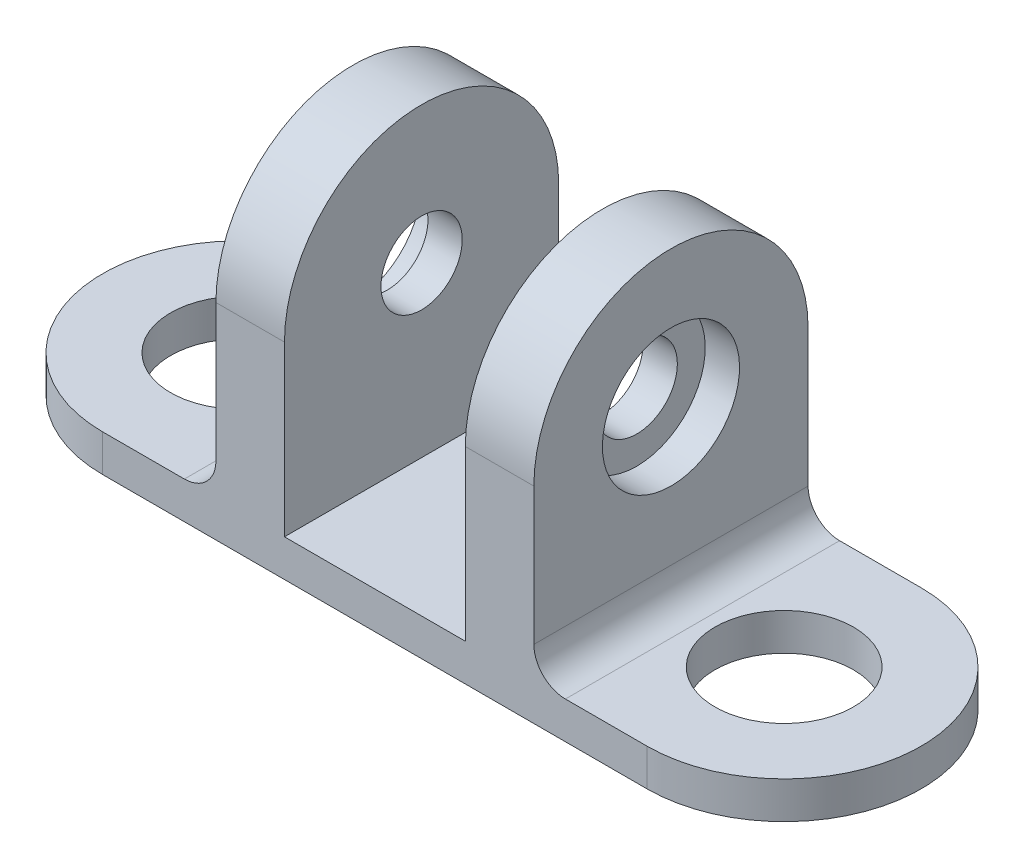
ISO-10303-21;
HEADER;
FILE_DESCRIPTION(('STEP AP214'),'2;1');
FILE_NAME('part.step','',(''),(''),'','','');
FILE_SCHEMA(('AUTOMOTIVE_DESIGN { 1 0 10303 214 1 1 1 1 }'));
ENDSEC;
DATA;
#1=APPLICATION_CONTEXT('core data for automotive mechanical design processes');
#2=APPLICATION_PROTOCOL_DEFINITION('international standard','automotive_design',2000,#1);
#3=PRODUCT_CONTEXT('',#1,'mechanical');
#4=PRODUCT('Part','Part','',(#3));
#5=PRODUCT_RELATED_PRODUCT_CATEGORY('part','',(#4));
#6=PRODUCT_DEFINITION_FORMATION('','',#4);
#7=PRODUCT_DEFINITION_CONTEXT('part definition',#1,'design');
#8=PRODUCT_DEFINITION('design','',#6,#7);
#9=PRODUCT_DEFINITION_SHAPE('','',#8);
#10=(LENGTH_UNIT() NAMED_UNIT(*) SI_UNIT(.MILLI.,.METRE.));
#11=(NAMED_UNIT(*) PLANE_ANGLE_UNIT() SI_UNIT($,.RADIAN.));
#12=(NAMED_UNIT(*) SI_UNIT($,.STERADIAN.) SOLID_ANGLE_UNIT());
#13=UNCERTAINTY_MEASURE_WITH_UNIT(LENGTH_MEASURE(1.E-05),#10,'distance_accuracy_value','');
#14=(GEOMETRIC_REPRESENTATION_CONTEXT(3) GLOBAL_UNCERTAINTY_ASSIGNED_CONTEXT((#13)) GLOBAL_UNIT_ASSIGNED_CONTEXT((#10,
#11,#12)) REPRESENTATION_CONTEXT('',''));
#15=CARTESIAN_POINT('',(0.,0.,0.));
#16=DIRECTION('',(0.,0.,1.));
#17=DIRECTION('',(1.,0.,0.));
#18=AXIS2_PLACEMENT_3D('',#15,#16,#17);
#19=CARTESIAN_POINT('',(-14.9812864248725,15.,0.));
#20=DIRECTION('',(1.,0.,0.));
#21=DIRECTION('',(0.,1.,0.));
#22=AXIS2_PLACEMENT_3D('',#19,#20,#21);
#23=CYLINDRICAL_SURFACE('',#22,2.965);
#24=CARTESIAN_POINT('',(6.595,15.,0.));
#25=DIRECTION('',(-1.,0.,0.));
#26=DIRECTION('',(0.,0.,1.));
#27=AXIS2_PLACEMENT_3D('',#24,#25,#26);
#28=CIRCLE('',#27,2.965);
#29=CARTESIAN_POINT('',(6.595,15.,2.965));
#30=VERTEX_POINT('',#29);
#31=EDGE_CURVE('E267',#30,#30,#28,.T.);
#32=ORIENTED_EDGE('',*,*,#31,.T.);
#33=EDGE_LOOP('',(#32));
#34=FACE_BOUND('',#33,.T.);
#35=CARTESIAN_POINT('',(9.095,15.,0.));
#36=DIRECTION('',(1.,0.,0.));
#37=DIRECTION('',(0.,1.,0.));
#38=AXIS2_PLACEMENT_3D('',#35,#36,#37);
#39=CIRCLE('',#38,2.965);
#40=CARTESIAN_POINT('',(9.095,17.965,0.));
#41=VERTEX_POINT('',#40);
#42=EDGE_CURVE('E43',#41,#41,#39,.T.);
#43=ORIENTED_EDGE('',*,*,#42,.T.);
#44=EDGE_LOOP('',(#43));
#45=FACE_BOUND('',#44,.T.);
#46=ADVANCED_FACE('F39',(#34,#45),#23,.F.);
#47=CARTESIAN_POINT('',(1.79128642487246,15.,0.));
#48=DIRECTION('',(-1.,0.,0.));
#49=DIRECTION('',(0.,-1.,0.));
#50=AXIS2_PLACEMENT_3D('',#47,#48,#49);
#51=CYLINDRICAL_SURFACE('',#50,2.965);
#52=CARTESIAN_POINT('',(-6.595,15.,0.));
#53=DIRECTION('',(1.,0.,0.));
#54=DIRECTION('',(0.,0.,-1.));
#55=AXIS2_PLACEMENT_3D('',#52,#53,#54);
#56=CIRCLE('',#55,2.965);
#57=CARTESIAN_POINT('',(-6.595,15.,-2.965));
#58=VERTEX_POINT('',#57);
#59=EDGE_CURVE('E155',#58,#58,#56,.F.);
#60=ORIENTED_EDGE('',*,*,#59,.F.);
#61=EDGE_LOOP('',(#60));
#62=FACE_BOUND('',#61,.T.);
#63=CARTESIAN_POINT('',(-9.095,15.,0.));
#64=DIRECTION('',(-1.,0.,0.));
#65=DIRECTION('',(0.,-1.,0.));
#66=AXIS2_PLACEMENT_3D('',#63,#64,#65);
#67=CIRCLE('',#66,2.965);
#68=CARTESIAN_POINT('',(-9.095,12.035,0.));
#69=VERTEX_POINT('',#68);
#70=EDGE_CURVE('E258',#69,#69,#67,.F.);
#71=ORIENTED_EDGE('',*,*,#70,.F.);
#72=EDGE_LOOP('',(#71));
#73=FACE_BOUND('',#72,.T.);
#74=ADVANCED_FACE('F313',(#62,#73),#51,.F.);
#75=CARTESIAN_POINT('',(-19.85,2.7,0.));
#76=DIRECTION('',(0.,1.,0.));
#77=DIRECTION('',(0.,0.,1.));
#78=AXIS2_PLACEMENT_3D('',#75,#76,#77);
#79=PLANE('',#78);
#80=DIRECTION('',(-1.,0.,0.));
#81=VECTOR('',#80,1.);
#82=CARTESIAN_POINT('',(-19.85,2.7,-10.));
#83=LINE('',#82,#81);
#84=CARTESIAN_POINT('',(19.85,2.7,-10.));
#85=VERTEX_POINT('',#84);
#86=CARTESIAN_POINT('',(13.895,2.7,-10.));
#87=VERTEX_POINT('',#86);
#88=EDGE_CURVE('E222',#85,#87,#83,.T.);
#89=ORIENTED_EDGE('',*,*,#88,.T.);
#90=DIRECTION('',(0.,0.,1.));
#91=VECTOR('',#90,1.);
#92=CARTESIAN_POINT('',(13.895,2.7,10.));
#93=LINE('',#92,#91);
#94=CARTESIAN_POINT('',(13.895,2.7,10.));
#95=VERTEX_POINT('',#94);
#96=EDGE_CURVE('E243',#87,#95,#93,.T.);
#97=ORIENTED_EDGE('',*,*,#96,.T.);
#98=DIRECTION('',(1.,0.,0.));
#99=VECTOR('',#98,1.);
#100=CARTESIAN_POINT('',(-19.85,2.7,10.));
#101=LINE('',#100,#99);
#102=CARTESIAN_POINT('',(19.85,2.7,10.));
#103=VERTEX_POINT('',#102);
#104=EDGE_CURVE('E213',#95,#103,#101,.T.);
#105=ORIENTED_EDGE('',*,*,#104,.T.);
#106=CARTESIAN_POINT('',(19.85,2.7,0.));
#107=DIRECTION('',(0.,1.,0.));
#108=DIRECTION('',(0.,0.,1.));
#109=AXIS2_PLACEMENT_3D('',#106,#107,#108);
#110=CIRCLE('',#109,10.);
#111=EDGE_CURVE('E220',#103,#85,#110,.T.);
#112=ORIENTED_EDGE('',*,*,#111,.T.);
#113=EDGE_LOOP('',(#89,#97,#105,#112));
#114=FACE_BOUND('',#113,.T.);
#115=CARTESIAN_POINT('',(19.85,2.7,0.));
#116=DIRECTION('',(0.,1.,0.));
#117=DIRECTION('',(0.,0.,1.));
#118=AXIS2_PLACEMENT_3D('',#115,#116,#117);
#119=CIRCLE('',#118,5.05);
#120=CARTESIAN_POINT('',(19.85,2.7,-5.05));
#121=VERTEX_POINT('',#120);
#122=EDGE_CURVE('E196',#121,#121,#119,.T.);
#123=ORIENTED_EDGE('',*,*,#122,.F.);
#124=EDGE_LOOP('',(#123));
#125=FACE_BOUND('',#124,.T.);
#126=ADVANCED_FACE('F317',(#114,#125),#79,.T.);
#127=DIRECTION('',(0.,0.,1.));
#128=VECTOR('',#127,1.);
#129=CARTESIAN_POINT('',(6.595,2.7,-23.2774244490413));
#130=LINE('',#129,#128);
#131=CARTESIAN_POINT('',(6.595,2.7,-10.));
#132=VERTEX_POINT('',#131);
#133=CARTESIAN_POINT('',(6.595,2.7,10.));
#134=VERTEX_POINT('',#133);
#135=EDGE_CURVE('E163',#132,#134,#130,.T.);
#136=ORIENTED_EDGE('',*,*,#135,.F.);
#137=CARTESIAN_POINT('',(-6.595,2.7,-10.));
#138=VERTEX_POINT('',#137);
#139=EDGE_CURVE('E223',#132,#138,#83,.T.);
#140=ORIENTED_EDGE('',*,*,#139,.T.);
#141=DIRECTION('',(0.,0.,1.));
#142=VECTOR('',#141,1.);
#143=CARTESIAN_POINT('',(-6.595,2.7,-23.2774244490413));
#144=LINE('',#143,#142);
#145=CARTESIAN_POINT('',(-6.595,2.7,10.));
#146=VERTEX_POINT('',#145);
#147=EDGE_CURVE('E184',#138,#146,#144,.T.);
#148=ORIENTED_EDGE('',*,*,#147,.T.);
#149=EDGE_CURVE('E217',#146,#134,#101,.T.);
#150=ORIENTED_EDGE('',*,*,#149,.T.);
#151=EDGE_LOOP('',(#136,#140,#148,#150));
#152=FACE_BOUND('',#151,.T.);
#153=ADVANCED_FACE('F358',(#152),#79,.T.);
#154=CARTESIAN_POINT('',(-19.85,2.7,10.));
#155=VERTEX_POINT('',#154);
#156=CARTESIAN_POINT('',(-13.895,2.7,10.));
#157=VERTEX_POINT('',#156);
#158=EDGE_CURVE('E214',#155,#157,#101,.T.);
#159=ORIENTED_EDGE('',*,*,#158,.T.);
#160=DIRECTION('',(0.,0.,1.));
#161=VECTOR('',#160,1.);
#162=CARTESIAN_POINT('',(-13.895,2.7,-10.));
#163=LINE('',#162,#161);
#164=CARTESIAN_POINT('',(-13.895,2.7,-10.));
#165=VERTEX_POINT('',#164);
#166=EDGE_CURVE('E62',#157,#165,#163,.F.);
#167=ORIENTED_EDGE('',*,*,#166,.T.);
#168=CARTESIAN_POINT('',(-19.85,2.7,-10.));
#169=VERTEX_POINT('',#168);
#170=EDGE_CURVE('E219',#165,#169,#83,.T.);
#171=ORIENTED_EDGE('',*,*,#170,.T.);
#172=CARTESIAN_POINT('',(-19.85,2.7,0.));
#173=DIRECTION('',(0.,1.,0.));
#174=DIRECTION('',(0.,0.,1.));
#175=AXIS2_PLACEMENT_3D('',#172,#173,#174);
#176=CIRCLE('',#175,10.);
#177=EDGE_CURVE('E209',#169,#155,#176,.T.);
#178=ORIENTED_EDGE('',*,*,#177,.T.);
#179=EDGE_LOOP('',(#159,#167,#171,#178));
#180=FACE_BOUND('',#179,.T.);
#181=CARTESIAN_POINT('',(-19.85,2.7,0.));
#182=DIRECTION('',(0.,1.,0.));
#183=DIRECTION('',(0.,0.,1.));
#184=AXIS2_PLACEMENT_3D('',#181,#182,#183);
#185=CIRCLE('',#184,5.05);
#186=CARTESIAN_POINT('',(-19.85,2.7,-5.05));
#187=VERTEX_POINT('',#186);
#188=EDGE_CURVE('E204',#187,#187,#185,.T.);
#189=ORIENTED_EDGE('',*,*,#188,.F.);
#190=EDGE_LOOP('',(#189));
#191=FACE_BOUND('',#190,.T.);
#192=ADVANCED_FACE('F352',(#180,#191),#79,.T.);
#193=CARTESIAN_POINT('',(-19.85,0.,0.));
#194=DIRECTION('',(0.,1.,0.));
#195=DIRECTION('',(0.,0.,1.));
#196=AXIS2_PLACEMENT_3D('',#193,#194,#195);
#197=PLANE('',#196);
#198=CARTESIAN_POINT('',(-19.85,0.,0.));
#199=DIRECTION('',(0.,1.,0.));
#200=DIRECTION('',(0.,0.,1.));
#201=AXIS2_PLACEMENT_3D('',#198,#199,#200);
#202=CIRCLE('',#201,10.);
#203=CARTESIAN_POINT('',(-19.85,0.,-10.));
#204=VERTEX_POINT('',#203);
#205=CARTESIAN_POINT('',(-19.85,0.,10.));
#206=VERTEX_POINT('',#205);
#207=EDGE_CURVE('E210',#204,#206,#202,.T.);
#208=ORIENTED_EDGE('',*,*,#207,.F.);
#209=DIRECTION('',(-1.,0.,0.));
#210=VECTOR('',#209,1.);
#211=CARTESIAN_POINT('',(-19.85,0.,-10.));
#212=LINE('',#211,#210);
#213=CARTESIAN_POINT('',(19.85,0.,-10.));
#214=VERTEX_POINT('',#213);
#215=EDGE_CURVE('E212',#214,#204,#212,.T.);
#216=ORIENTED_EDGE('',*,*,#215,.F.);
#217=CARTESIAN_POINT('',(19.85,0.,0.));
#218=DIRECTION('',(0.,1.,0.));
#219=DIRECTION('',(0.,0.,1.));
#220=AXIS2_PLACEMENT_3D('',#217,#218,#219);
#221=CIRCLE('',#220,10.);
#222=CARTESIAN_POINT('',(19.85,0.,10.));
#223=VERTEX_POINT('',#222);
#224=EDGE_CURVE('E230',#223,#214,#221,.T.);
#225=ORIENTED_EDGE('',*,*,#224,.F.);
#226=DIRECTION('',(1.,0.,0.));
#227=VECTOR('',#226,1.);
#228=CARTESIAN_POINT('',(-19.85,0.,10.));
#229=LINE('',#228,#227);
#230=EDGE_CURVE('E229',#206,#223,#229,.T.);
#231=ORIENTED_EDGE('',*,*,#230,.F.);
#232=EDGE_LOOP('',(#208,#216,#225,#231));
#233=FACE_BOUND('',#232,.T.);
#234=CARTESIAN_POINT('',(-19.85,0.,0.));
#235=DIRECTION('',(0.,1.,0.));
#236=DIRECTION('',(0.,0.,1.));
#237=AXIS2_PLACEMENT_3D('',#234,#235,#236);
#238=CIRCLE('',#237,5.05);
#239=CARTESIAN_POINT('',(-19.85,0.,-5.05));
#240=VERTEX_POINT('',#239);
#241=EDGE_CURVE('E203',#240,#240,#238,.T.);
#242=ORIENTED_EDGE('',*,*,#241,.T.);
#243=EDGE_LOOP('',(#242));
#244=FACE_BOUND('',#243,.T.);
#245=CARTESIAN_POINT('',(19.85,0.,0.));
#246=DIRECTION('',(0.,1.,0.));
#247=DIRECTION('',(0.,0.,1.));
#248=AXIS2_PLACEMENT_3D('',#245,#246,#247);
#249=CIRCLE('',#248,5.05);
#250=CARTESIAN_POINT('',(19.85,0.,-5.05));
#251=VERTEX_POINT('',#250);
#252=EDGE_CURVE('E197',#251,#251,#249,.T.);
#253=ORIENTED_EDGE('',*,*,#252,.T.);
#254=EDGE_LOOP('',(#253));
#255=FACE_BOUND('',#254,.T.);
#256=ADVANCED_FACE('F355',(#233,#244,#255),#197,.F.);
#257=CARTESIAN_POINT('',(-19.85,2.7,0.));
#258=DIRECTION('',(0.,-1.,0.));
#259=DIRECTION('',(0.,0.,-1.));
#260=AXIS2_PLACEMENT_3D('',#257,#258,#259);
#261=CYLINDRICAL_SURFACE('',#260,10.);
#262=ORIENTED_EDGE('',*,*,#207,.T.);
#263=DIRECTION('',(0.,-1.,0.));
#264=VECTOR('',#263,1.);
#265=CARTESIAN_POINT('',(-19.85,2.7,10.));
#266=LINE('',#265,#264);
#267=EDGE_CURVE('E241',#155,#206,#266,.T.);
#268=ORIENTED_EDGE('',*,*,#267,.F.);
#269=ORIENTED_EDGE('',*,*,#177,.F.);
#270=DIRECTION('',(0.,-1.,0.));
#271=VECTOR('',#270,1.);
#272=CARTESIAN_POINT('',(-19.85,2.7,-10.));
#273=LINE('',#272,#271);
#274=EDGE_CURVE('E221',#169,#204,#273,.T.);
#275=ORIENTED_EDGE('',*,*,#274,.T.);
#276=EDGE_LOOP('',(#262,#268,#269,#275));
#277=FACE_BOUND('',#276,.T.);
#278=ADVANCED_FACE('F360',(#277),#261,.T.);
#279=CARTESIAN_POINT('',(-19.85,2.7,10.));
#280=DIRECTION('',(0.,0.,-1.));
#281=DIRECTION('',(-1.,0.,0.));
#282=AXIS2_PLACEMENT_3D('',#279,#280,#281);
#283=PLANE('',#282);
#284=DIRECTION('',(0.,-1.,0.));
#285=VECTOR('',#284,1.);
#286=CARTESIAN_POINT('',(-11.595,15.,10.));
#287=LINE('',#286,#285);
#288=CARTESIAN_POINT('',(-11.595,15.,10.));
#289=VERTEX_POINT('',#288);
#290=CARTESIAN_POINT('',(-11.595,5.,10.));
#291=VERTEX_POINT('',#290);
#292=EDGE_CURVE('E194',#289,#291,#287,.T.);
#293=ORIENTED_EDGE('',*,*,#292,.T.);
#294=CARTESIAN_POINT('',(-13.895,5.,10.));
#295=DIRECTION('',(0.,0.,-1.));
#296=DIRECTION('',(-1.,0.,0.));
#297=AXIS2_PLACEMENT_3D('',#294,#295,#296);
#298=CIRCLE('',#297,2.3);
#299=EDGE_CURVE('E48',#291,#157,#298,.T.);
#300=ORIENTED_EDGE('',*,*,#299,.T.);
#301=ORIENTED_EDGE('',*,*,#158,.F.);
#302=ORIENTED_EDGE('',*,*,#267,.T.);
#303=ORIENTED_EDGE('',*,*,#230,.T.);
#304=DIRECTION('',(0.,-1.,0.));
#305=VECTOR('',#304,1.);
#306=CARTESIAN_POINT('',(19.85,2.7,10.));
#307=LINE('',#306,#305);
#308=EDGE_CURVE('E236',#103,#223,#307,.T.);
#309=ORIENTED_EDGE('',*,*,#308,.F.);
#310=ORIENTED_EDGE('',*,*,#104,.F.);
#311=CARTESIAN_POINT('',(13.895,5.,10.));
#312=DIRECTION('',(0.,0.,-1.));
#313=DIRECTION('',(-1.,0.,0.));
#314=AXIS2_PLACEMENT_3D('',#311,#312,#313);
#315=CIRCLE('',#314,2.3);
#316=CARTESIAN_POINT('',(11.595,5.,10.));
#317=VERTEX_POINT('',#316);
#318=EDGE_CURVE('E162',#95,#317,#315,.T.);
#319=ORIENTED_EDGE('',*,*,#318,.T.);
#320=DIRECTION('',(0.,-1.,0.));
#321=VECTOR('',#320,1.);
#322=CARTESIAN_POINT('',(11.595,15.,10.));
#323=LINE('',#322,#321);
#324=CARTESIAN_POINT('',(11.595,15.,10.));
#325=VERTEX_POINT('',#324);
#326=EDGE_CURVE('E145',#325,#317,#323,.T.);
#327=ORIENTED_EDGE('',*,*,#326,.F.);
#328=DIRECTION('',(1.,0.,0.));
#329=VECTOR('',#328,1.);
#330=CARTESIAN_POINT('',(6.595,15.,10.));
#331=LINE('',#330,#329);
#332=CARTESIAN_POINT('',(6.595,15.,10.));
#333=VERTEX_POINT('',#332);
#334=EDGE_CURVE('E154',#333,#325,#331,.T.);
#335=ORIENTED_EDGE('',*,*,#334,.F.);
#336=DIRECTION('',(0.,1.,0.));
#337=VECTOR('',#336,1.);
#338=CARTESIAN_POINT('',(6.595,2.7,10.));
#339=LINE('',#338,#337);
#340=EDGE_CURVE('E157',#134,#333,#339,.T.);
#341=ORIENTED_EDGE('',*,*,#340,.F.);
#342=ORIENTED_EDGE('',*,*,#149,.F.);
#343=DIRECTION('',(0.,1.,0.));
#344=VECTOR('',#343,1.);
#345=CARTESIAN_POINT('',(-6.595,2.7,10.));
#346=LINE('',#345,#344);
#347=CARTESIAN_POINT('',(-6.595,15.,10.));
#348=VERTEX_POINT('',#347);
#349=EDGE_CURVE('E180',#146,#348,#346,.T.);
#350=ORIENTED_EDGE('',*,*,#349,.T.);
#351=DIRECTION('',(-1.,0.,0.));
#352=VECTOR('',#351,1.);
#353=CARTESIAN_POINT('',(-6.595,15.,10.));
#354=LINE('',#353,#352);
#355=EDGE_CURVE('E188',#348,#289,#354,.T.);
#356=ORIENTED_EDGE('',*,*,#355,.T.);
#357=EDGE_LOOP('',(#293,#300,#301,#302,#303,#309,#310,#319,#327,#335,#341,#342,#350,#356));
#358=FACE_BOUND('',#357,.T.);
#359=ADVANCED_FACE('F161',(#358),#283,.F.);
#360=CARTESIAN_POINT('',(19.85,2.7,0.));
#361=DIRECTION('',(0.,-1.,0.));
#362=DIRECTION('',(0.,0.,-1.));
#363=AXIS2_PLACEMENT_3D('',#360,#361,#362);
#364=CYLINDRICAL_SURFACE('',#363,10.);
#365=ORIENTED_EDGE('',*,*,#224,.T.);
#366=DIRECTION('',(0.,-1.,0.));
#367=VECTOR('',#366,1.);
#368=CARTESIAN_POINT('',(19.85,2.7,-10.));
#369=LINE('',#368,#367);
#370=EDGE_CURVE('E231',#85,#214,#369,.T.);
#371=ORIENTED_EDGE('',*,*,#370,.F.);
#372=ORIENTED_EDGE('',*,*,#111,.F.);
#373=ORIENTED_EDGE('',*,*,#308,.T.);
#374=EDGE_LOOP('',(#365,#371,#372,#373));
#375=FACE_BOUND('',#374,.T.);
#376=ADVANCED_FACE('F361',(#375),#364,.T.);
#377=CARTESIAN_POINT('',(-19.85,2.7,-10.));
#378=DIRECTION('',(0.,0.,1.));
#379=DIRECTION('',(1.,0.,0.));
#380=AXIS2_PLACEMENT_3D('',#377,#378,#379);
#381=PLANE('',#380);
#382=DIRECTION('',(0.,-1.,0.));
#383=VECTOR('',#382,1.);
#384=CARTESIAN_POINT('',(-6.595,2.7,-10.));
#385=LINE('',#384,#383);
#386=CARTESIAN_POINT('',(-6.595,15.,-10.));
#387=VERTEX_POINT('',#386);
#388=EDGE_CURVE('E186',#387,#138,#385,.T.);
#389=ORIENTED_EDGE('',*,*,#388,.T.);
#390=ORIENTED_EDGE('',*,*,#139,.F.);
#391=DIRECTION('',(0.,-1.,0.));
#392=VECTOR('',#391,1.);
#393=CARTESIAN_POINT('',(6.595,2.7,-10.));
#394=LINE('',#393,#392);
#395=CARTESIAN_POINT('',(6.595,15.,-10.));
#396=VERTEX_POINT('',#395);
#397=EDGE_CURVE('E171',#396,#132,#394,.T.);
#398=ORIENTED_EDGE('',*,*,#397,.F.);
#399=DIRECTION('',(-1.,0.,0.));
#400=VECTOR('',#399,1.);
#401=CARTESIAN_POINT('',(6.595,15.,-10.));
#402=LINE('',#401,#400);
#403=CARTESIAN_POINT('',(11.595,15.,-10.));
#404=VERTEX_POINT('',#403);
#405=EDGE_CURVE('E170',#404,#396,#402,.T.);
#406=ORIENTED_EDGE('',*,*,#405,.F.);
#407=DIRECTION('',(0.,1.,0.));
#408=VECTOR('',#407,1.);
#409=CARTESIAN_POINT('',(11.595,15.,-10.));
#410=LINE('',#409,#408);
#411=CARTESIAN_POINT('',(11.595,5.,-10.));
#412=VERTEX_POINT('',#411);
#413=EDGE_CURVE('E150',#412,#404,#410,.T.);
#414=ORIENTED_EDGE('',*,*,#413,.F.);
#415=CARTESIAN_POINT('',(13.895,5.,-10.));
#416=DIRECTION('',(0.,0.,1.));
#417=DIRECTION('',(1.,0.,0.));
#418=AXIS2_PLACEMENT_3D('',#415,#416,#417);
#419=CIRCLE('',#418,2.3);
#420=EDGE_CURVE('E255',#412,#87,#419,.T.);
#421=ORIENTED_EDGE('',*,*,#420,.T.);
#422=ORIENTED_EDGE('',*,*,#88,.F.);
#423=ORIENTED_EDGE('',*,*,#370,.T.);
#424=ORIENTED_EDGE('',*,*,#215,.T.);
#425=ORIENTED_EDGE('',*,*,#274,.F.);
#426=ORIENTED_EDGE('',*,*,#170,.F.);
#427=CARTESIAN_POINT('',(-13.895,5.,-10.));
#428=DIRECTION('',(0.,0.,1.));
#429=DIRECTION('',(1.,0.,0.));
#430=AXIS2_PLACEMENT_3D('',#427,#428,#429);
#431=CIRCLE('',#430,2.3);
#432=CARTESIAN_POINT('',(-11.595,5.,-10.));
#433=VERTEX_POINT('',#432);
#434=EDGE_CURVE('E11',#165,#433,#431,.T.);
#435=ORIENTED_EDGE('',*,*,#434,.T.);
#436=DIRECTION('',(0.,1.,0.));
#437=VECTOR('',#436,1.);
#438=CARTESIAN_POINT('',(-11.595,15.,-10.));
#439=LINE('',#438,#437);
#440=CARTESIAN_POINT('',(-11.595,15.,-10.));
#441=VERTEX_POINT('',#440);
#442=EDGE_CURVE('E181',#433,#441,#439,.T.);
#443=ORIENTED_EDGE('',*,*,#442,.T.);
#444=DIRECTION('',(1.,0.,0.));
#445=VECTOR('',#444,1.);
#446=CARTESIAN_POINT('',(-6.595,15.,-10.));
#447=LINE('',#446,#445);
#448=EDGE_CURVE('E176',#441,#387,#447,.T.);
#449=ORIENTED_EDGE('',*,*,#448,.T.);
#450=EDGE_LOOP('',(#389,#390,#398,#406,#414,#421,#422,#423,#424,#425,#426,#435,#443,#449));
#451=FACE_BOUND('',#450,.T.);
#452=ADVANCED_FACE('F286',(#451),#381,.F.);
#453=CARTESIAN_POINT('',(-19.85,2.7,0.));
#454=DIRECTION('',(0.,-1.,0.));
#455=DIRECTION('',(0.,0.,-1.));
#456=AXIS2_PLACEMENT_3D('',#453,#454,#455);
#457=CYLINDRICAL_SURFACE('',#456,5.05);
#458=CARTESIAN_POINT('',(-19.85,2.7,-5.05));
#459=CARTESIAN_POINT('',(-19.85,2.671875,-5.05));
#460=CARTESIAN_POINT('',(-19.85,2.64375,-5.05));
#461=CARTESIAN_POINT('',(-19.85,2.5875,-5.05));
#462=CARTESIAN_POINT('',(-19.85,2.559375,-5.05));
#463=CARTESIAN_POINT('',(-19.85,2.503125,-5.05));
#464=CARTESIAN_POINT('',(-19.85,2.475,-5.05));
#465=CARTESIAN_POINT('',(-19.85,2.41875,-5.05));
#466=CARTESIAN_POINT('',(-19.85,2.390625,-5.05));
#467=CARTESIAN_POINT('',(-19.85,2.334375,-5.05));
#468=CARTESIAN_POINT('',(-19.85,2.30625,-5.05));
#469=CARTESIAN_POINT('',(-19.85,2.25,-5.05));
#470=CARTESIAN_POINT('',(-19.85,2.221875,-5.05));
#471=CARTESIAN_POINT('',(-19.85,2.165625,-5.05));
#472=CARTESIAN_POINT('',(-19.85,2.1375,-5.05));
#473=CARTESIAN_POINT('',(-19.85,2.08125,-5.05));
#474=CARTESIAN_POINT('',(-19.85,2.053125,-5.05));
#475=CARTESIAN_POINT('',(-19.85,1.996875,-5.05));
#476=CARTESIAN_POINT('',(-19.85,1.96875,-5.05));
#477=CARTESIAN_POINT('',(-19.85,1.9125,-5.05));
#478=CARTESIAN_POINT('',(-19.85,1.884375,-5.05));
#479=CARTESIAN_POINT('',(-19.85,1.828125,-5.05));
#480=CARTESIAN_POINT('',(-19.85,1.8,-5.05));
#481=CARTESIAN_POINT('',(-19.85,1.74375,-5.05));
#482=CARTESIAN_POINT('',(-19.85,1.715625,-5.05));
#483=CARTESIAN_POINT('',(-19.85,1.659375,-5.05));
#484=CARTESIAN_POINT('',(-19.85,1.63125,-5.05));
#485=CARTESIAN_POINT('',(-19.85,1.575,-5.05));
#486=CARTESIAN_POINT('',(-19.85,1.546875,-5.05));
#487=CARTESIAN_POINT('',(-19.85,1.490625,-5.05));
#488=CARTESIAN_POINT('',(-19.85,1.4625,-5.05));
#489=CARTESIAN_POINT('',(-19.85,1.40625,-5.05));
#490=CARTESIAN_POINT('',(-19.85,1.378125,-5.05));
#491=CARTESIAN_POINT('',(-19.85,1.321875,-5.05));
#492=CARTESIAN_POINT('',(-19.85,1.29375,-5.05));
#493=CARTESIAN_POINT('',(-19.85,1.2375,-5.05));
#494=CARTESIAN_POINT('',(-19.85,1.209375,-5.05));
#495=CARTESIAN_POINT('',(-19.85,1.153125,-5.05));
#496=CARTESIAN_POINT('',(-19.85,1.125,-5.05));
#497=CARTESIAN_POINT('',(-19.85,1.06875,-5.05));
#498=CARTESIAN_POINT('',(-19.85,1.040625,-5.05));
#499=CARTESIAN_POINT('',(-19.85,0.984375,-5.05));
#500=CARTESIAN_POINT('',(-19.85,0.956249999999999,-5.05));
#501=CARTESIAN_POINT('',(-19.85,0.899999999999999,-5.05));
#502=CARTESIAN_POINT('',(-19.85,0.871875,-5.05));
#503=CARTESIAN_POINT('',(-19.85,0.815624999999999,-5.05));
#504=CARTESIAN_POINT('',(-19.85,0.787499999999999,-5.05));
#505=CARTESIAN_POINT('',(-19.85,0.73125,-5.05));
#506=CARTESIAN_POINT('',(-19.85,0.703125,-5.05));
#507=CARTESIAN_POINT('',(-19.85,0.646875,-5.05));
#508=CARTESIAN_POINT('',(-19.85,0.61875,-5.05));
#509=CARTESIAN_POINT('',(-19.85,0.5625,-5.05));
#510=CARTESIAN_POINT('',(-19.85,0.534375,-5.05));
#511=CARTESIAN_POINT('',(-19.85,0.478125,-5.05));
#512=CARTESIAN_POINT('',(-19.85,0.45,-5.05));
#513=CARTESIAN_POINT('',(-19.85,0.39375,-5.05));
#514=CARTESIAN_POINT('',(-19.85,0.365625,-5.05));
#515=CARTESIAN_POINT('',(-19.85,0.309375,-5.05));
#516=CARTESIAN_POINT('',(-19.85,0.28125,-5.05));
#517=CARTESIAN_POINT('',(-19.85,0.225,-5.05));
#518=CARTESIAN_POINT('',(-19.85,0.196875,-5.05));
#519=CARTESIAN_POINT('',(-19.85,0.140625,-5.05));
#520=CARTESIAN_POINT('',(-19.85,0.1125,-5.05));
#521=CARTESIAN_POINT('',(-19.85,0.0562499999999997,-5.05));
#522=CARTESIAN_POINT('',(-19.85,0.0281249999999996,-5.05));
#523=CARTESIAN_POINT('',(-19.85,0.,-5.05));
#524=B_SPLINE_CURVE_WITH_KNOTS('',3,(#458,#459,#460,#461,#462,#463,#464,#465,#466,#467,#468,
#469,#470,#471,#472,#473,#474,#475,#476,#477,#478,#479,#480,#481,#482,#483,#484,#485,#486,#487,
#488,#489,#490,#491,#492,#493,#494,#495,#496,#497,#498,#499,#500,#501,#502,#503,#504,#505,#506,
#507,#508,#509,#510,#511,#512,#513,#514,#515,#516,#517,#518,#519,#520,#521,#522,#523),
.UNSPECIFIED.,.F.,.F.,(4,2,2,2,2,2,2,2,2,2,2,2,2,2,2,2,2,2,2,2,2,2,2,2,2,2,2,2,2,2,2,2,4),(0.,
0.0843750000000003,0.16875,0.253125,0.3375,0.421875,0.50625,0.590625,0.675,0.759375,0.84375,
0.928125000000001,1.0125,1.096875,1.18125,1.265625,1.35,1.434375,1.51875,1.603125,1.6875,
1.771875,1.85625,1.940625,2.025,2.109375,2.19375,2.278125,2.3625,2.446875,2.53125,2.615625,2.7),.UNSPECIFIED.);
#525=EDGE_CURVE('BSEAM350',#187,#240,#524,.T.);
#526=ORIENTED_EDGE('',*,*,#188,.T.);
#527=ORIENTED_EDGE('',*,*,#241,.F.);
#528=ORIENTED_EDGE('',*,*,#525,.T.);
#529=ORIENTED_EDGE('',*,*,#525,.F.);
#530=EDGE_LOOP('',(#526,#528,#527,#529));
#531=FACE_BOUND('',#530,.T.);
#532=ADVANCED_FACE('F350',(#531),#457,.F.);
#533=CARTESIAN_POINT('',(19.85,2.7,0.));
#534=DIRECTION('',(0.,-1.,0.));
#535=DIRECTION('',(0.,0.,-1.));
#536=AXIS2_PLACEMENT_3D('',#533,#534,#535);
#537=CYLINDRICAL_SURFACE('',#536,5.05);
#538=CARTESIAN_POINT('',(19.85,2.7,-5.05));
#539=CARTESIAN_POINT('',(19.85,2.671875,-5.05));
#540=CARTESIAN_POINT('',(19.85,2.64375,-5.05));
#541=CARTESIAN_POINT('',(19.85,2.5875,-5.05));
#542=CARTESIAN_POINT('',(19.85,2.559375,-5.05));
#543=CARTESIAN_POINT('',(19.85,2.503125,-5.05));
#544=CARTESIAN_POINT('',(19.85,2.475,-5.05));
#545=CARTESIAN_POINT('',(19.85,2.41875,-5.05));
#546=CARTESIAN_POINT('',(19.85,2.390625,-5.05));
#547=CARTESIAN_POINT('',(19.85,2.334375,-5.05));
#548=CARTESIAN_POINT('',(19.85,2.30625,-5.05));
#549=CARTESIAN_POINT('',(19.85,2.25,-5.05));
#550=CARTESIAN_POINT('',(19.85,2.221875,-5.05));
#551=CARTESIAN_POINT('',(19.85,2.165625,-5.05));
#552=CARTESIAN_POINT('',(19.85,2.1375,-5.05));
#553=CARTESIAN_POINT('',(19.85,2.08125,-5.05));
#554=CARTESIAN_POINT('',(19.85,2.053125,-5.05));
#555=CARTESIAN_POINT('',(19.85,1.996875,-5.05));
#556=CARTESIAN_POINT('',(19.85,1.96875,-5.05));
#557=CARTESIAN_POINT('',(19.85,1.9125,-5.05));
#558=CARTESIAN_POINT('',(19.85,1.884375,-5.05));
#559=CARTESIAN_POINT('',(19.85,1.828125,-5.05));
#560=CARTESIAN_POINT('',(19.85,1.8,-5.05));
#561=CARTESIAN_POINT('',(19.85,1.74375,-5.05));
#562=CARTESIAN_POINT('',(19.85,1.715625,-5.05));
#563=CARTESIAN_POINT('',(19.85,1.659375,-5.05));
#564=CARTESIAN_POINT('',(19.85,1.63125,-5.05));
#565=CARTESIAN_POINT('',(19.85,1.575,-5.05));
#566=CARTESIAN_POINT('',(19.85,1.546875,-5.05));
#567=CARTESIAN_POINT('',(19.85,1.490625,-5.05));
#568=CARTESIAN_POINT('',(19.85,1.4625,-5.05));
#569=CARTESIAN_POINT('',(19.85,1.40625,-5.05));
#570=CARTESIAN_POINT('',(19.85,1.378125,-5.05));
#571=CARTESIAN_POINT('',(19.85,1.321875,-5.05));
#572=CARTESIAN_POINT('',(19.85,1.29375,-5.05));
#573=CARTESIAN_POINT('',(19.85,1.2375,-5.05));
#574=CARTESIAN_POINT('',(19.85,1.209375,-5.05));
#575=CARTESIAN_POINT('',(19.85,1.153125,-5.05));
#576=CARTESIAN_POINT('',(19.85,1.125,-5.05));
#577=CARTESIAN_POINT('',(19.85,1.06875,-5.05));
#578=CARTESIAN_POINT('',(19.85,1.040625,-5.05));
#579=CARTESIAN_POINT('',(19.85,0.984375,-5.05));
#580=CARTESIAN_POINT('',(19.85,0.956249999999999,-5.05));
#581=CARTESIAN_POINT('',(19.85,0.899999999999999,-5.05));
#582=CARTESIAN_POINT('',(19.85,0.871875,-5.05));
#583=CARTESIAN_POINT('',(19.85,0.815624999999999,-5.05));
#584=CARTESIAN_POINT('',(19.85,0.787499999999999,-5.05));
#585=CARTESIAN_POINT('',(19.85,0.73125,-5.05));
#586=CARTESIAN_POINT('',(19.85,0.703125,-5.05));
#587=CARTESIAN_POINT('',(19.85,0.646875,-5.05));
#588=CARTESIAN_POINT('',(19.85,0.61875,-5.05));
#589=CARTESIAN_POINT('',(19.85,0.5625,-5.05));
#590=CARTESIAN_POINT('',(19.85,0.534375,-5.05));
#591=CARTESIAN_POINT('',(19.85,0.478125,-5.05));
#592=CARTESIAN_POINT('',(19.85,0.45,-5.05));
#593=CARTESIAN_POINT('',(19.85,0.39375,-5.05));
#594=CARTESIAN_POINT('',(19.85,0.365625,-5.05));
#595=CARTESIAN_POINT('',(19.85,0.309375,-5.05));
#596=CARTESIAN_POINT('',(19.85,0.28125,-5.05));
#597=CARTESIAN_POINT('',(19.85,0.225,-5.05));
#598=CARTESIAN_POINT('',(19.85,0.196875,-5.05));
#599=CARTESIAN_POINT('',(19.85,0.140625,-5.05));
#600=CARTESIAN_POINT('',(19.85,0.1125,-5.05));
#601=CARTESIAN_POINT('',(19.85,0.0562499999999997,-5.05));
#602=CARTESIAN_POINT('',(19.85,0.0281249999999996,-5.05));
#603=CARTESIAN_POINT('',(19.85,0.,-5.05));
#604=B_SPLINE_CURVE_WITH_KNOTS('',3,(#538,#539,#540,#541,#542,#543,#544,#545,#546,#547,#548,
#549,#550,#551,#552,#553,#554,#555,#556,#557,#558,#559,#560,#561,#562,#563,#564,#565,#566,#567,
#568,#569,#570,#571,#572,#573,#574,#575,#576,#577,#578,#579,#580,#581,#582,#583,#584,#585,#586,
#587,#588,#589,#590,#591,#592,#593,#594,#595,#596,#597,#598,#599,#600,#601,#602,#603),
.UNSPECIFIED.,.F.,.F.,(4,2,2,2,2,2,2,2,2,2,2,2,2,2,2,2,2,2,2,2,2,2,2,2,2,2,2,2,2,2,2,2,4),(0.,
0.0843750000000003,0.16875,0.253125,0.3375,0.421875,0.50625,0.590625,0.675,0.759375,0.84375,
0.928125000000001,1.0125,1.096875,1.18125,1.265625,1.35,1.434375,1.51875,1.603125,1.6875,
1.771875,1.85625,1.940625,2.025,2.109375,2.19375,2.278125,2.3625,2.446875,2.53125,2.615625,2.7),.UNSPECIFIED.);
#605=EDGE_CURVE('BSEAM343',#121,#251,#604,.T.);
#606=ORIENTED_EDGE('',*,*,#122,.T.);
#607=ORIENTED_EDGE('',*,*,#252,.F.);
#608=ORIENTED_EDGE('',*,*,#605,.T.);
#609=ORIENTED_EDGE('',*,*,#605,.F.);
#610=EDGE_LOOP('',(#606,#608,#607,#609));
#611=FACE_BOUND('',#610,.T.);
#612=ADVANCED_FACE('F343',(#611),#537,.F.);
#613=CARTESIAN_POINT('',(-11.595,15.,-23.2774244490413));
#614=DIRECTION('',(-1.,0.,0.));
#615=DIRECTION('',(0.,-1.,0.));
#616=AXIS2_PLACEMENT_3D('',#613,#614,#615);
#617=PLANE('',#616);
#618=CARTESIAN_POINT('',(-11.595,15.,0.));
#619=DIRECTION('',(-1.,0.,0.));
#620=DIRECTION('',(0.,-1.,0.));
#621=AXIS2_PLACEMENT_3D('',#618,#619,#620);
#622=CIRCLE('',#621,5.);
#623=CARTESIAN_POINT('',(-11.595,10.,0.));
#624=VERTEX_POINT('',#623);
#625=EDGE_CURVE('E262',#624,#624,#622,.T.);
#626=ORIENTED_EDGE('',*,*,#625,.F.);
#627=EDGE_LOOP('',(#626));
#628=FACE_BOUND('',#627,.T.);
#629=ORIENTED_EDGE('',*,*,#442,.F.);
#630=DIRECTION('',(0.,0.,1.));
#631=VECTOR('',#630,1.);
#632=CARTESIAN_POINT('',(-11.595,5.,10.));
#633=LINE('',#632,#631);
#634=EDGE_CURVE('E250',#433,#291,#633,.T.);
#635=ORIENTED_EDGE('',*,*,#634,.T.);
#636=ORIENTED_EDGE('',*,*,#292,.F.);
#637=CARTESIAN_POINT('',(-11.595,15.,0.));
#638=DIRECTION('',(-1.,0.,0.));
#639=DIRECTION('',(0.,1.,0.));
#640=AXIS2_PLACEMENT_3D('',#637,#638,#639);
#641=CIRCLE('',#640,10.);
#642=EDGE_CURVE('E173',#289,#441,#641,.T.);
#643=ORIENTED_EDGE('',*,*,#642,.T.);
#644=EDGE_LOOP('',(#629,#635,#636,#643));
#645=FACE_BOUND('',#644,.T.);
#646=ADVANCED_FACE('F296',(#628,#645),#617,.T.);
#647=CARTESIAN_POINT('',(-6.595,2.7,-23.2774244490413));
#648=DIRECTION('',(1.,0.,0.));
#649=DIRECTION('',(0.,0.,-1.));
#650=AXIS2_PLACEMENT_3D('',#647,#648,#649);
#651=PLANE('',#650);
#652=ORIENTED_EDGE('',*,*,#59,.T.);
#653=EDGE_LOOP('',(#652));
#654=FACE_BOUND('',#653,.T.);
#655=ORIENTED_EDGE('',*,*,#388,.F.);
#656=CARTESIAN_POINT('',(-6.595,15.,0.));
#657=DIRECTION('',(1.,0.,0.));
#658=DIRECTION('',(0.,0.,-1.));
#659=AXIS2_PLACEMENT_3D('',#656,#657,#658);
#660=CIRCLE('',#659,10.);
#661=EDGE_CURVE('E179',#348,#387,#660,.F.);
#662=ORIENTED_EDGE('',*,*,#661,.F.);
#663=ORIENTED_EDGE('',*,*,#349,.F.);
#664=ORIENTED_EDGE('',*,*,#147,.F.);
#665=EDGE_LOOP('',(#655,#662,#663,#664));
#666=FACE_BOUND('',#665,.T.);
#667=ADVANCED_FACE('F285',(#654,#666),#651,.T.);
#668=CARTESIAN_POINT('',(15.7656797749979,15.,0.));
#669=DIRECTION('',(-1.,0.,0.));
#670=DIRECTION('',(0.,-1.,0.));
#671=AXIS2_PLACEMENT_3D('',#668,#669,#670);
#672=CYLINDRICAL_SURFACE('',#671,10.);
#673=ORIENTED_EDGE('',*,*,#355,.F.);
#674=ORIENTED_EDGE('',*,*,#661,.T.);
#675=ORIENTED_EDGE('',*,*,#448,.F.);
#676=ORIENTED_EDGE('',*,*,#642,.F.);
#677=EDGE_LOOP('',(#673,#674,#675,#676));
#678=FACE_BOUND('',#677,.T.);
#679=ADVANCED_FACE('F287',(#678),#672,.T.);
#680=CARTESIAN_POINT('',(11.595,15.,-23.2774244490413));
#681=DIRECTION('',(1.,0.,0.));
#682=DIRECTION('',(0.,-1.,0.));
#683=AXIS2_PLACEMENT_3D('',#680,#681,#682);
#684=PLANE('',#683);
#685=CARTESIAN_POINT('',(11.595,15.,0.));
#686=DIRECTION('',(-1.,0.,0.));
#687=DIRECTION('',(0.,-1.,0.));
#688=AXIS2_PLACEMENT_3D('',#685,#686,#687);
#689=CIRCLE('',#688,5.);
#690=CARTESIAN_POINT('',(11.595,10.,0.));
#691=VERTEX_POINT('',#690);
#692=EDGE_CURVE('E476',#691,#691,#689,.T.);
#693=ORIENTED_EDGE('',*,*,#692,.T.);
#694=EDGE_LOOP('',(#693));
#695=FACE_BOUND('',#694,.T.);
#696=ORIENTED_EDGE('',*,*,#326,.T.);
#697=DIRECTION('',(0.,0.,1.));
#698=VECTOR('',#697,1.);
#699=CARTESIAN_POINT('',(11.595,5.,-10.));
#700=LINE('',#699,#698);
#701=EDGE_CURVE('E249',#317,#412,#700,.F.);
#702=ORIENTED_EDGE('',*,*,#701,.T.);
#703=ORIENTED_EDGE('',*,*,#413,.T.);
#704=CARTESIAN_POINT('',(11.595,15.,0.));
#705=DIRECTION('',(-1.,0.,0.));
#706=DIRECTION('',(0.,1.,0.));
#707=AXIS2_PLACEMENT_3D('',#704,#705,#706);
#708=CIRCLE('',#707,10.);
#709=EDGE_CURVE('E136',#325,#404,#708,.T.);
#710=ORIENTED_EDGE('',*,*,#709,.F.);
#711=EDGE_LOOP('',(#696,#702,#703,#710));
#712=FACE_BOUND('',#711,.T.);
#713=ADVANCED_FACE('F142',(#695,#712),#684,.T.);
#714=CARTESIAN_POINT('',(6.595,2.7,-23.2774244490413));
#715=DIRECTION('',(-1.,0.,0.));
#716=DIRECTION('',(0.,0.,-1.));
#717=AXIS2_PLACEMENT_3D('',#714,#715,#716);
#718=PLANE('',#717);
#719=ORIENTED_EDGE('',*,*,#31,.F.);
#720=EDGE_LOOP('',(#719));
#721=FACE_BOUND('',#720,.T.);
#722=ORIENTED_EDGE('',*,*,#397,.T.);
#723=ORIENTED_EDGE('',*,*,#135,.T.);
#724=ORIENTED_EDGE('',*,*,#340,.T.);
#725=CARTESIAN_POINT('',(6.595,15.,0.));
#726=DIRECTION('',(1.,0.,0.));
#727=DIRECTION('',(0.,0.,-1.));
#728=AXIS2_PLACEMENT_3D('',#725,#726,#727);
#729=CIRCLE('',#728,10.);
#730=EDGE_CURVE('E151',#333,#396,#729,.F.);
#731=ORIENTED_EDGE('',*,*,#730,.T.);
#732=EDGE_LOOP('',(#722,#723,#724,#731));
#733=FACE_BOUND('',#732,.T.);
#734=ADVANCED_FACE('F280',(#721,#733),#718,.T.);
#735=CARTESIAN_POINT('',(-15.7656797749979,15.,0.));
#736=DIRECTION('',(1.,0.,0.));
#737=DIRECTION('',(0.,-1.,0.));
#738=AXIS2_PLACEMENT_3D('',#735,#736,#737);
#739=CYLINDRICAL_SURFACE('',#738,10.);
#740=ORIENTED_EDGE('',*,*,#334,.T.);
#741=ORIENTED_EDGE('',*,*,#709,.T.);
#742=ORIENTED_EDGE('',*,*,#405,.T.);
#743=ORIENTED_EDGE('',*,*,#730,.F.);
#744=EDGE_LOOP('',(#740,#741,#742,#743));
#745=FACE_BOUND('',#744,.T.);
#746=ADVANCED_FACE('F156',(#745),#739,.T.);
#747=CARTESIAN_POINT('',(13.895,5.,0.));
#748=DIRECTION('',(0.,0.,-1.));
#749=DIRECTION('',(-1.,0.,0.));
#750=AXIS2_PLACEMENT_3D('',#747,#748,#749);
#751=CYLINDRICAL_SURFACE('',#750,2.3);
#752=ORIENTED_EDGE('',*,*,#420,.F.);
#753=ORIENTED_EDGE('',*,*,#701,.F.);
#754=ORIENTED_EDGE('',*,*,#318,.F.);
#755=ORIENTED_EDGE('',*,*,#96,.F.);
#756=EDGE_LOOP('',(#752,#753,#754,#755));
#757=FACE_BOUND('',#756,.T.);
#758=ADVANCED_FACE('F303',(#757),#751,.F.);
#759=CARTESIAN_POINT('',(-13.895,5.,-23.2774244490413));
#760=DIRECTION('',(0.,0.,-1.));
#761=DIRECTION('',(-1.,0.,0.));
#762=AXIS2_PLACEMENT_3D('',#759,#760,#761);
#763=CYLINDRICAL_SURFACE('',#762,2.3);
#764=ORIENTED_EDGE('',*,*,#434,.F.);
#765=ORIENTED_EDGE('',*,*,#166,.F.);
#766=ORIENTED_EDGE('',*,*,#299,.F.);
#767=ORIENTED_EDGE('',*,*,#634,.F.);
#768=EDGE_LOOP('',(#764,#765,#766,#767));
#769=FACE_BOUND('',#768,.T.);
#770=ADVANCED_FACE('F41',(#769),#763,.F.);
#771=CARTESIAN_POINT('',(-9.095,15.,0.));
#772=DIRECTION('',(-1.,0.,0.));
#773=DIRECTION('',(0.,-1.,0.));
#774=AXIS2_PLACEMENT_3D('',#771,#772,#773);
#775=PLANE('',#774);
#776=CARTESIAN_POINT('',(-9.095,15.,0.));
#777=DIRECTION('',(-1.,0.,0.));
#778=DIRECTION('',(0.,-1.,0.));
#779=AXIS2_PLACEMENT_3D('',#776,#777,#778);
#780=CIRCLE('',#779,5.);
#781=CARTESIAN_POINT('',(-9.095,10.,0.));
#782=VERTEX_POINT('',#781);
#783=EDGE_CURVE('E256',#782,#782,#780,.T.);
#784=ORIENTED_EDGE('',*,*,#783,.T.);
#785=EDGE_LOOP('',(#784));
#786=FACE_BOUND('',#785,.T.);
#787=ORIENTED_EDGE('',*,*,#70,.T.);
#788=EDGE_LOOP('',(#787));
#789=FACE_BOUND('',#788,.T.);
#790=ADVANCED_FACE('F300',(#786,#789),#775,.T.);
#791=CARTESIAN_POINT('',(-9.095,15.,0.));
#792=DIRECTION('',(-1.,0.,0.));
#793=DIRECTION('',(0.,-1.,0.));
#794=AXIS2_PLACEMENT_3D('',#791,#792,#793);
#795=CYLINDRICAL_SURFACE('',#794,5.);
#796=ORIENTED_EDGE('',*,*,#783,.F.);
#797=EDGE_LOOP('',(#796));
#798=FACE_BOUND('',#797,.T.);
#799=ORIENTED_EDGE('',*,*,#625,.T.);
#800=EDGE_LOOP('',(#799));
#801=FACE_BOUND('',#800,.T.);
#802=ADVANCED_FACE('F307',(#798,#801),#795,.F.);
#803=CARTESIAN_POINT('',(9.095,15.,0.));
#804=DIRECTION('',(1.,0.,0.));
#805=DIRECTION('',(0.,1.,0.));
#806=AXIS2_PLACEMENT_3D('',#803,#804,#805);
#807=CYLINDRICAL_SURFACE('',#806,5.);
#808=CARTESIAN_POINT('',(9.095,15.,0.));
#809=DIRECTION('',(-1.,0.,0.));
#810=DIRECTION('',(0.,-1.,0.));
#811=AXIS2_PLACEMENT_3D('',#808,#809,#810);
#812=CIRCLE('',#811,5.);
#813=CARTESIAN_POINT('',(9.095,10.,0.));
#814=VERTEX_POINT('',#813);
#815=EDGE_CURVE('E480',#814,#814,#812,.T.);
#816=ORIENTED_EDGE('',*,*,#815,.T.);
#817=EDGE_LOOP('',(#816));
#818=FACE_BOUND('',#817,.T.);
#819=ORIENTED_EDGE('',*,*,#692,.F.);
#820=EDGE_LOOP('',(#819));
#821=FACE_BOUND('',#820,.T.);
#822=ADVANCED_FACE('F324',(#818,#821),#807,.F.);
#823=CARTESIAN_POINT('',(9.095,15.,0.));
#824=DIRECTION('',(1.,0.,0.));
#825=DIRECTION('',(0.,-1.,0.));
#826=AXIS2_PLACEMENT_3D('',#823,#824,#825);
#827=PLANE('',#826);
#828=ORIENTED_EDGE('',*,*,#42,.F.);
#829=EDGE_LOOP('',(#828));
#830=FACE_BOUND('',#829,.T.);
#831=ORIENTED_EDGE('',*,*,#815,.F.);
#832=EDGE_LOOP('',(#831));
#833=FACE_BOUND('',#832,.T.);
#834=ADVANCED_FACE('F461',(#830,#833),#827,.T.);
#835=CLOSED_SHELL('',(#46,#74,#126,#153,#192,#256,#278,#359,#376,#452,#532,#612,#646,#667,#679,
#713,#734,#746,#758,#770,#790,#802,#822,#834));
#836=MANIFOLD_SOLID_BREP('B2',#835);
#837=ADVANCED_BREP_SHAPE_REPRESENTATION('',(#18,#836),#14);
#838=SHAPE_DEFINITION_REPRESENTATION(#9,#837);
ENDSEC;
END-ISO-10303-21;
